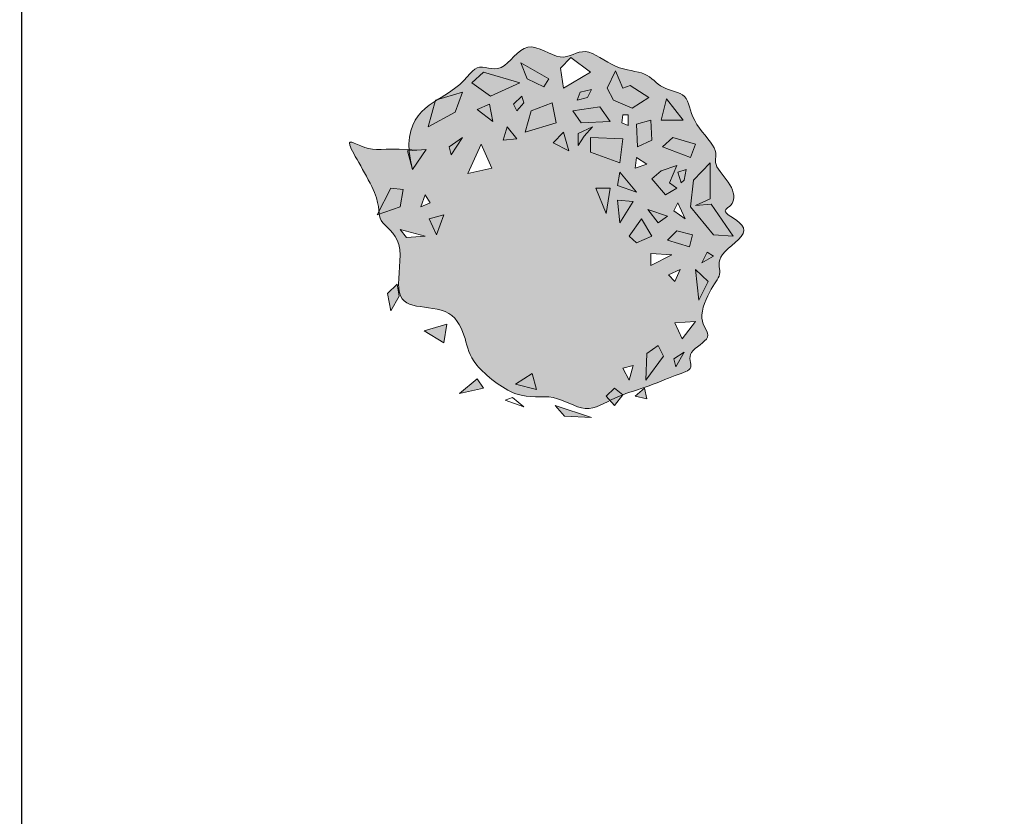
# Model space of a CAD drawing. Units: metres. Extents: x 4298.5 to 4325.2, y 2075 to 2095.8.
# Tile 29 of 35: x 4320.314 to 4321.936, y 2082.247 to 2083.561. Entities that reach past the tile are written whole.
import ezdxf

# ---------------------------------------------------------------- set-up
doc = ezdxf.new("R2010")
doc.units = ezdxf.units.M
doc.layers.add('A-ANNO-DIMS', color=2, linetype='Continuous', lineweight=18)
doc.layers.add('L-PLNT', color=94, linetype='Continuous', lineweight=13)
doc.layers.add('L-PLNT-PATT', color=116, linetype='Continuous', lineweight=13, true_color=0x13823e)
doc.styles.get("Standard").update_dxf_attribs({"font": 'arial.ttf'})
doc.dimstyles.get("Standard").update_dxf_attribs({"dimtxt": 0.18, "dimasz": 0.18, "dimexe": 0.18, "dimexo": 0.0625, "dimgap": 0.09, "dimtad": 0, "dimtih": 1, "dimtoh": 1, "dimdec": 4, "dimzin": 0, "dimdsep": 46, "dimtxsty": 'Standard', "dimcen": 0.09, "dimadec": 0, "dimazin": 0, "dimtfac": 1, "dimtdec": 4, "dimtofl": 0, "dimtmove": 0, "dimatfit": 3, "dimfxl": 1, "dimtolj": 1, "dimtzin": 0, "dimarcsym": 0})

# ---------------------------------------------------------------- blocks, each defined once
blk = doc.blocks.new('*U9')
for points in [[(-2.003, 11.656), (-1.598, 10.618), (-0.518, 10.099), (-0.181, 10.618), (-0.788, 10.964)], [(1.237, 12.003), (0.562, 11.31), (0.764, 10.013), (2.519, 11.051)], [(-4.432, 11.051), (-5.175, 10.359), (-3.96, 9.493), (-2.07, 10.359)], [(4.139, 11.137), (3.599, 10.013), (4.004, 9.234), (5.218, 8.715), (6.298, 9.407), (5.083, 10.186), (4.611, 10.013)], [(-5.782, 9.753), (-7.537, 9.234), (-8.009, 7.504), (-6.255, 8.455)], [(2.586, 9.926), (1.844, 9.753), (1.642, 9.234), (2.316, 9.407)], [(-4.837, 8.628), (-3.825, 7.85), (-4.027, 8.974)], [(-1.935, 9.493), (-2.475, 8.974), (-2.273, 8.542), (-1.8, 9.061)], [(0.022, 9.061), (-1.328, 8.542), (-1.733, 7.157), (0.292, 7.763)], [(7.446, 9.32), (7.108, 7.936), (8.525, 7.936)], [(1.372, 8.542), (3.126, 8.801), (3.801, 7.85), (1.912, 7.763)], [(4.611, 8.282), (4.544, 7.763), (4.949, 7.59), (4.949, 8.282)], [(6.433, 7.936), (5.488, 7.676), (5.556, 6.206), (6.501, 6.638)], [(-2.88, 7.504), (-3.15, 6.638), (-2.273, 6.725)], [(0.764, 7.157), (0.089, 6.465), (1.102, 5.946)], [(1.709, 6.292), (1.709, 7.071), (2.654, 7.504), (2.114, 6.898)], [(-5.782, 6.811), (-6.659, 6.206), (-6.524, 5.687)], [(2.519, 6.811), (2.519, 5.86), (4.409, 5.167), (4.611, 6.725)], [(7.851, 6.811), (7.176, 6.206), (8.998, 5.514), (9.335, 6.379)], [(-8.144, 6.033), (-9.359, 5.946), (-9.022, 4.735)], [(-4.567, 6.379), (-5.445, 4.475), (-3.892, 4.821)], [(5.488, 5.514), (5.421, 4.821), (6.163, 5.081)], [(10.28, 5.167), (9.2, 4.043), (8.998, 2.312), (10.482, 0.495), (11.765, 0.409), (10.348, 2.485), (9.335, 2.399), (10.28, 2.831)], [(4.409, 4.562), (4.274, 3.697), (5.488, 3.264)], [(8.12, 4.994), (7.108, 4.648), (6.501, 4.129), (7.378, 3.091), (8.12, 3.524), (7.648, 3.87)], [(8.728, 4.735), (8.188, 4.562), (8.39, 3.87), (8.593, 4.043)], [(-11.316, 1.793), (-9.831, 2.312), (-9.629, 3.437), (-10.439, 3.524)], [(3.531, 1.88), (2.856, 3.524), (3.801, 3.524)], [(-8.212, 3.091), (-8.482, 2.312), (-7.874, 2.572)], [(4.274, 2.745), (5.286, 2.658), (4.409, 1.274)], [(8.188, 2.572), (7.918, 2.053), (8.66, 1.534)], [(7.513, 1.707), (6.906, 1.274), (6.231, 2.139)], [(-6.997, 1.793), (-7.942, 1.534), (-7.469, 0.495)], [(5.826, 1.534), (5.016, 0.409), (5.488, -0.024), (6.501, 0.409)], [(-8.212, 0.409), (-9.426, 0.322), (-9.831, 0.841)], [(8.12, 0.755), (7.513, 0.149), (8.93, -0.283), (9.133, 0.495)], [(10.078, -0.629), (9.74, -1.322), (10.482, -0.889)], [(7.783, -0.803), (6.433, -1.495), (6.433, -0.716)], [(8.323, -1.754), (7.985, -2.533), (7.581, -2.1)], [(9.335, -1.754), (9.538, -3.744), (10.145, -2.533)], [(-10.034, -2.706), (-10.641, -3.312), (-10.439, -4.436), (-9.899, -3.485)], [(-8.279, -5.734), (-6.794, -5.302), (-6.997, -6.513)], [(9.335, -5.129), (8.458, -6.253), (7.985, -5.215)], [(6.096, -8.935), (6.163, -7.205), (6.906, -6.686), (7.243, -7.378)], [(8.053, -8.07), (8.593, -7.118), (7.918, -7.551)], [(5.286, -7.984), (4.611, -8.157), (5.016, -8.935)], [(-4.837, -8.849), (-4.432, -9.454), (-5.985, -9.801)], [(-2.34, -9.195), (-1.26, -8.503), (-0.99, -9.541)], [(4.071, -9.454), (3.531, -9.974), (4.071, -10.579), (4.611, -9.887)], [(6.028, -9.454), (5.421, -9.974), (6.163, -10.147)], [(-2.543, -10.06), (-3.015, -10.233), (-1.8, -10.666)], [(0.224, -10.579), (0.832, -11.272), (2.586, -11.358)]]:
    blk.add_lwpolyline(points, close=True)
blk = doc.blocks.new('*D47')
at = {"layer": 'A-ANNO-DIMS', "color": 0, "lineweight": -2, "transparency": 16777216}
for p, q in [((4300.4306, 2084.4956), (4300.4306, 2074.9896)), ((4322.8106, 2084.4956), (4322.8106, 2074.9896)), ((4300.6106, 2075.1696), (4311.2252, 2075.1696)), ((4322.6306, 2075.1696), (4312.016, 2075.1696))]:
    blk.add_line(p, q, dxfattribs=at)
at = {"layer": 'A-ANNO-DIMS', "color": 0, "transparency": 16777216}
for points in [[(4300.6106, 2075.1996), (4300.6106, 2075.1396), (4300.4306, 2075.1696)], [(4322.6306, 2075.1996), (4322.6306, 2075.1396), (4322.8106, 2075.1696)]]:
    blk.add_solid(points, dxfattribs=at)
at = {"layer": 'Defpoints', "color": 0, "transparency": 16777216}
for p in [(4300.4306, 2084.5581), (4322.8106, 2084.5581), (4322.8106, 2075.1696)]:
    blk.add_point(p, dxfattribs=at)
at = {"layer": 'A-ANNO-DIMS', "color": 0, "transparency": 16777216, "insert": (4311.6206, 2075.1696), "char_height": 0.18, "attachment_point": 5}
blk.add_mtext('\\A1;22.38', dxfattribs=at)
blk = doc.blocks.new('*D48')
at = {"layer": 'A-ANNO-DIMS', "color": 0, "lineweight": -2, "transparency": 16777216}
for p, q in [((4310.1831, 2094.4781), (4324.7671, 2094.4781)), ((4324.5871, 2094.2981), (4324.5871, 2085.585)), ((4324.5871, 2076.5081), (4324.5871, 2085.2212)), ((4316.8731, 2076.3281), (4324.7671, 2076.3281))]:
    blk.add_line(p, q, dxfattribs=at)
at = {"layer": 'A-ANNO-DIMS', "color": 0, "transparency": 16777216}
for points in [[(4324.5571, 2094.2981), (4324.6171, 2094.2981), (4324.5871, 2094.4781)], [(4324.5571, 2076.5081), (4324.6171, 2076.5081), (4324.5871, 2076.3281)]]:
    blk.add_solid(points, dxfattribs=at)
at = {"layer": 'Defpoints', "color": 0, "transparency": 16777216}
for p in [(4310.1206, 2094.4781), (4316.8106, 2076.3281), (4324.5871, 2076.3281)]:
    blk.add_point(p, dxfattribs=at)
at = {"layer": 'A-ANNO-DIMS', "color": 0, "transparency": 16777216, "insert": (4324.5871, 2085.4031), "char_height": 0.18, "attachment_point": 5}
blk.add_mtext('\\A1;18.15', dxfattribs=at)
blk = doc.blocks.new('*D55')
at = {"layer": 'A-ANNO-DIMS', "color": 0, "lineweight": -2, "transparency": 16777216}
for p, q in [((4320.3167, 2084.4996), (4320.3167, 2074.9896)), ((4322.8106, 2084.4956), (4322.8106, 2074.9896)), ((4320.4967, 2075.1696), (4321.1688, 2075.1696)), ((4322.6306, 2075.1696), (4321.9585, 2075.1696))]:
    blk.add_line(p, q, dxfattribs=at)
at = {"layer": 'A-ANNO-DIMS', "color": 0, "transparency": 16777216}
for points in [[(4320.4967, 2075.1996), (4320.4967, 2075.1396), (4320.3167, 2075.1696)], [(4322.6306, 2075.1996), (4322.6306, 2075.1396), (4322.8106, 2075.1696)]]:
    blk.add_solid(points, dxfattribs=at)
at = {"layer": 'Defpoints', "color": 0, "transparency": 16777216}
for p in [(4320.3167, 2084.5621), (4322.8106, 2084.5581), (4322.8106, 2075.1696)]:
    blk.add_point(p, dxfattribs=at)
at = {"layer": 'A-ANNO-DIMS', "color": 0, "transparency": 16777216, "insert": (4321.5636, 2075.1696), "char_height": 0.18, "attachment_point": 5}
blk.add_mtext('\\A1;2.494', dxfattribs=at)

msp = doc.modelspace()

# ---------------------------------------------------------------- hatches: boundary and pattern name
at = {"layer": 'L-PLNT-PATT'}
h = msp.add_hatch(color=256, dxfattribs=at)
h.dxf.hatch_style = 1
edge = h.paths.add_edge_path()
edge.add_spline(control_points=[(4321.2862, 2082.9328), (4321.2888, 2082.9341), (4321.3075, 2082.9435), (4321.3433, 2082.9532), (4321.3978, 2082.9765), (4321.4271, 2082.9841), (4321.4084, 2083.0126), (4321.461, 2083.0368), (4321.4273, 2083.0631), (4321.4543, 2083.1228), (4321.473, 2083.1423), (4321.4564, 2083.1708), (4321.5306, 2083.2156), (4321.4607, 2083.2452), (4321.4933, 2083.2529), (4321.4894, 2083.288), (4321.4513, 2083.3246), (4321.4698, 2083.3439), (4321.4168, 2083.3949), (4321.4168, 2083.441), (4321.3689, 2083.4443), (4321.3485, 2083.4762), (4321.2953, 2083.4762), (4321.2429, 2083.5216), (4321.2082, 2083.4845), (4321.1475, 2083.5353), (4321.1076, 2083.4653), (4321.063, 2083.4952), (4321.0487, 2083.4559), (4321.0084, 2083.4328), (4321.002, 2083.4289)], knot_values=[0.818571, 0.818571, 0.818571, 0.818571, 0.97924, 1.97924, 2.97924, 3.97924, 4.97924, 5.97924, 6.97924, 7.97924, 8.97924, 9.97924, 10.97924, 11.97924, 12.97924, 13.97924, 14.97924, 15.97924, 16.97924, 17.97924, 18.97924, 19.97924, 20.97924, 21.97924, 22.97924, 23.97924, 24.97924, 25.97924, 26.97924, 27.16067, 27.16067, 27.16067, 27.16067], degree=3, periodic=0)
edge.add_line((4321.002, 2083.4289), (4321.0433, 2083.4411))
edge.add_line((4321.0433, 2083.4411), (4321.0313, 2083.4081))
edge.add_line((4321.0313, 2083.4081), (4320.9867, 2083.384))
edge.add_line((4320.9867, 2083.384), (4320.9983, 2083.4265))
edge.add_spline(control_points=[(4320.9983, 2083.4265), (4320.9757, 2083.4119), (4320.9524, 2083.3909), (4320.9551, 2083.3465)], knot_values=[0.141368, 0.141368, 0.141368, 0.141368, 0.783694, 0.783694, 0.783694, 0.783694], degree=3, periodic=0)
edge.add_spline(control_points=[(4320.9551, 2083.3465), (4320.9591, 2083.3463), (4320.9633, 2083.3459), (4320.9679, 2083.3455)], knot_values=[40.901028, 40.901028, 40.901028, 40.901028, 41, 41, 41, 41], degree=3, periodic=0)
edge.add_line((4320.9679, 2083.3455), (4320.9833, 2083.3466))
edge.add_line((4320.9833, 2083.3466), (4320.961, 2083.3136))
edge.add_line((4320.961, 2083.3136), (4320.9524, 2083.3444))
edge.add_line((4320.9524, 2083.3444), (4320.9552, 2083.3446))
edge.add_spline(control_points=[(4320.9553, 2083.3446), (4320.9552, 2083.3452), (4320.9552, 2083.3459), (4320.9551, 2083.3465)], knot_values=[0.13204, 0.13204, 0.13204, 0.13204, 0.141368, 0.141368, 0.141368, 0.141368], degree=3, periodic=0)
edge.add_spline(control_points=[(4320.9551, 2083.3465), (4320.9189, 2083.3489), (4320.8873, 2083.339), (4320.8353, 2083.381), (4320.9023, 2083.2785), (4320.9047, 2083.2516), (4320.9054, 2083.2441)], knot_values=[37.439141, 37.439141, 37.439141, 37.439141, 38.340169, 39.340169, 40.340169, 40.901028, 40.901028, 40.901028, 40.901028], degree=3, periodic=0)
edge.add_line((4320.9054, 2083.2441), (4320.925, 2083.2829))
edge.add_line((4320.925, 2083.2829), (4320.9456, 2083.2807))
edge.add_line((4320.9456, 2083.2807), (4320.9404, 2083.2521))
edge.add_line((4320.9404, 2083.2521), (4320.9058, 2083.24))
edge.add_spline(control_points=[(4320.9058, 2083.24), (4320.9063, 2083.236), (4320.9094, 2083.2225), (4320.9507, 2083.2015), (4320.9293, 2083.1043), (4320.9615, 2083.0854), (4321.0277, 2083.0854), (4321.0505, 2083.0317), (4321.054, 2082.9962), (4321.135, 2082.9301), (4321.1933, 2082.9469), (4321.2437, 2082.91), (4321.2728, 2082.926), (4321.2862, 2082.9328)], knot_values=[27.16067, 27.16067, 27.16067, 27.16067, 27.490087, 28.490087, 29.490087, 30.490087, 31.490087, 32.490087, 33.490087, 34.490087, 35.490087, 36.490087, 37.329418, 37.329418, 37.329418, 37.329418], degree=3, periodic=0)
edge.add_line((4321.2862, 2082.9328), (4321.2798, 2082.94))
edge.add_line((4321.2798, 2082.94), (4321.2935, 2082.9532))
edge.add_line((4321.2935, 2082.9532), (4321.3073, 2082.9422))
h.paths.add_polyline_path([(4321.2627, 2083.2829), (4321.2867, 2083.2829), (4321.2798, 2083.2411)], flags=16)
h.paths.add_polyline_path([(4321.2987, 2083.2631), (4321.3244, 2083.2609), (4321.3021, 2083.2257)], flags=16)
h.paths.add_polyline_path([(4321.0913, 2083.3158), (4321.0518, 2083.307), (4321.0741, 2083.3554)], flags=16)
h.paths.add_polyline_path([(4321.2181, 2083.3444), (4321.1924, 2083.3576), (4321.2095, 2083.3751)], flags=16)
h.paths.add_polyline_path([(4321.2987, 2083.2873), (4321.3021, 2083.3092), (4321.3295, 2083.2763)], flags=16)
h.paths.add_polyline_path([(4321.3175, 2083.2037), (4321.3381, 2083.2323), (4321.3553, 2083.2037), (4321.3295, 2083.1927)], flags=16)
h.paths.add_polyline_path([(4321.2541, 2083.3422), (4321.2541, 2083.3664), (4321.3073, 2083.3642), (4321.3021, 2083.3246)], flags=16)
h.paths.add_polyline_path([(4321.2335, 2083.3532), (4321.2335, 2083.373), (4321.2576, 2083.384), (4321.2438, 2083.3686)], flags=16)
h.paths.add_polyline_path([(4321.1324, 2083.3642), (4321.1101, 2083.362), (4321.117, 2083.384)], flags=16)
h.paths.add_polyline_path([(4321.1461, 2083.3751), (4321.1564, 2083.4103), (4321.1907, 2083.4235), (4321.1976, 2083.3905)], flags=16)
h.paths.add_polyline_path([(4321.0124, 2083.2389), (4321.0004, 2083.2059), (4320.9884, 2083.2323)], flags=16)
h.paths.add_polyline_path([(4321.3484, 2083.2477), (4321.381, 2083.2367), (4321.3656, 2083.2257)], flags=16)
h.paths.add_polyline_path([(4321.3278, 2083.3158), (4321.3295, 2083.3334), (4321.3467, 2083.3224)], flags=16)
h.paths.add_polyline_path([(4321.2387, 2083.3905), (4321.225, 2083.4103), (4321.2695, 2083.4169), (4321.2867, 2083.3927)], flags=16)
h.paths.add_polyline_path([(4321.3535, 2083.1752), (4321.3878, 2083.173), (4321.3535, 2083.1554)], flags=16)
h.paths.add_polyline_path([(4320.9901, 2083.2587), (4320.9747, 2083.2521), (4320.9816, 2083.2719)], flags=16)
h.paths.add_polyline_path([(4321.093, 2083.3927), (4321.0673, 2083.4125), (4321.0879, 2083.4213)], flags=16)
h.paths.add_polyline_path([(4321.0244, 2083.3378), (4321.021, 2083.351), (4321.0433, 2083.3664)], flags=16)
h.paths.add_polyline_path([(4321.1324, 2083.4103), (4321.1273, 2083.4213), (4321.141, 2083.4345), (4321.1444, 2083.4235)], flags=16)
h.paths.add_polyline_path([(4321.3553, 2083.2982), (4321.3707, 2083.3114), (4321.3964, 2083.3202), (4321.3844, 2083.2917), (4321.3964, 2083.2829), (4321.3775, 2083.2719)], flags=16)
h.paths.add_polyline_path([(4320.9816, 2083.2037), (4320.9507, 2083.2015), (4320.9404, 2083.2147)], flags=16)
h.paths.add_polyline_path([(4321.3313, 2083.351), (4321.3295, 2083.3883), (4321.3535, 2083.3949), (4321.3553, 2083.362)], flags=16)
h.paths.add_polyline_path([(4321.381, 2083.1971), (4321.3964, 2083.2125), (4321.4221, 2083.2059), (4321.417, 2083.1862)], flags=16)
h.paths.add_polyline_path([(4321.3056, 2083.3905), (4321.3073, 2083.4037), (4321.3158, 2083.4037), (4321.3158, 2083.3861)], flags=16)
h.paths.add_polyline_path([(4321.2318, 2083.4279), (4321.237, 2083.4411), (4321.2558, 2083.4455), (4321.249, 2083.4323)], flags=16)
h.paths.add_polyline_path([(4321.3913, 2083.2455), (4321.3981, 2083.2587), (4321.4101, 2083.2323)], flags=16)
h.paths.add_polyline_path([(4321.3827, 2083.14), (4321.4015, 2083.1488), (4321.393, 2083.129)], flags=16)
h.paths.add_polyline_path([(4321.177, 2083.4499), (4321.1496, 2083.4631), (4321.1393, 2083.4894), (4321.1701, 2083.4718), (4321.1855, 2083.4631)], flags=16)
h.paths.add_polyline_path([(4321.2095, 2083.4477), (4321.2044, 2083.4806), (4321.2216, 2083.4982), (4321.2541, 2083.4741)], flags=16)
h.paths.add_polyline_path([(4321.0896, 2083.4345), (4321.0587, 2083.4565), (4321.0776, 2083.4741), (4321.1376, 2083.4565)], flags=16)
h.paths.add_polyline_path([(4321.3724, 2083.351), (4321.3896, 2083.3664), (4321.4273, 2083.3554), (4321.4187, 2083.3334)], flags=16)
h.paths.add_polyline_path([(4321.2918, 2083.4279), (4321.2816, 2083.4477), (4321.2953, 2083.4762), (4321.3073, 2083.4477), (4321.3192, 2083.4521), (4321.3501, 2083.4323), (4321.3227, 2083.4147)], flags=16)
h.paths.add_polyline_path([(4321.4032, 2083.2917), (4321.3981, 2083.3092), (4321.4118, 2083.3136), (4321.4084, 2083.2961)], flags=16)
h.paths.add_polyline_path([(4321.4187, 2083.2521), (4321.4238, 2083.2961), (4321.4513, 2083.3246), (4321.4513, 2083.2653), (4321.4273, 2083.2543), (4321.453, 2083.2565), (4321.489, 2083.2037), (4321.4564, 2083.2059)], flags=16)
h.paths.add_polyline_path([(4321.1581, 2082.9774), (4321.165, 2082.951), (4321.1307, 2082.9598)], flags=16)
h.paths.add_polyline_path([(4321.3707, 2083.3949), (4321.3793, 2083.4301), (4321.4067, 2083.3949)], flags=16)
h.paths.add_polyline_path([(4321.4273, 2083.1488), (4321.4478, 2083.129), (4321.4324, 2083.0983)], flags=16)
h.paths.add_polyline_path([(4321.4375, 2083.1598), (4321.4461, 2083.1774), (4321.4564, 2083.1708)], flags=16)
h.paths.add_polyline_path([(4321.3073, 2082.9862), (4321.3244, 2082.9906), (4321.3175, 2082.9664)], flags=16)
h.paths.add_polyline_path([(4321.393, 2083.0609), (4321.4273, 2083.0631), (4321.405, 2083.0345)], flags=16)
h.paths.add_polyline_path([(4321.3467, 2083.0104), (4321.3656, 2083.0235), (4321.3741, 2083.006), (4321.345, 2082.9664)], flags=16)
h.paths.add_polyline_path([(4321.3913, 2083.0016), (4321.4084, 2083.0126), (4321.3947, 2082.9884)], flags=16)
h = msp.add_hatch(color=256, dxfattribs=at)
h.dxf.hatch_style = 1
h.paths.add_polyline_path([(4321.3021, 2083.3246), (4321.3073, 2083.3642), (4321.2541, 2083.3664), (4321.2541, 2083.3422)])
h.paths.add_polyline_path([(4321.3484, 2083.2477), (4321.3656, 2083.2257), (4321.381, 2083.2367)])
h.paths.add_polyline_path([(4321.3295, 2083.3883), (4321.3313, 2083.351), (4321.3553, 2083.362), (4321.3535, 2083.3949)])
h.paths.add_polyline_path([(4321.3501, 2083.4323), (4321.3192, 2083.4521), (4321.3073, 2083.4477), (4321.2953, 2083.4762), (4321.2816, 2083.4477), (4321.2918, 2083.4279), (4321.3227, 2083.4147)])
h.paths.add_polyline_path([(4321.1958, 2082.9247), (4321.2113, 2082.907), (4321.2558, 2082.9049)])
h.paths.add_polyline_path([(4321.177, 2083.4499), (4321.1855, 2083.4631), (4321.1701, 2083.4718), (4321.1393, 2083.4894), (4321.1496, 2083.4631)])
h.paths.add_polyline_path([(4321.0776, 2083.4741), (4321.0587, 2083.4565), (4321.0896, 2083.4345), (4321.1376, 2083.4565)])
h.paths.add_polyline_path([(4321.1564, 2083.4103), (4321.1461, 2083.3751), (4321.1976, 2083.3905), (4321.1907, 2083.4235)])
h.paths.add_polyline_path([(4321.1444, 2083.4235), (4321.141, 2083.4345), (4321.1273, 2083.4213), (4321.1324, 2083.4103)])
h.paths.add_polyline_path([(4321.117, 2083.384), (4321.1101, 2083.362), (4321.1324, 2083.3642)])
h.paths.add_polyline_path([(4321.093, 2083.3927), (4321.0879, 2083.4213), (4321.0673, 2083.4125)])
h.paths.add_polyline_path([(4320.9987, 2083.4279), (4320.9867, 2083.384), (4321.0313, 2083.4081), (4321.0433, 2083.4411)])
h.paths.add_polyline_path([(4321.0433, 2083.3664), (4321.021, 2083.351), (4321.0244, 2083.3378)])
h.paths.add_polyline_path([(4320.9524, 2083.3444), (4320.961, 2083.3136), (4320.9833, 2083.3466)])
h.paths.add_polyline_path([(4320.9027, 2083.2389), (4320.9404, 2083.2521), (4320.9456, 2083.2807), (4320.925, 2083.2829)])
h.paths.add_polyline_path([(4321.0124, 2083.2389), (4320.9884, 2083.2323), (4321.0004, 2083.2059)])
h.paths.add_polyline_path([(4320.9387, 2083.1048), (4320.9353, 2083.1246), (4320.9199, 2083.1092), (4320.925, 2083.0807)])
h.paths.add_polyline_path([(4321.0176, 2083.0587), (4320.9799, 2083.0477), (4321.0124, 2083.0279)])
h.paths.add_polyline_path([(4321.0381, 2082.9444), (4321.0776, 2082.9532), (4321.0673, 2082.9686)])
h.paths.add_polyline_path([(4321.1581, 2082.9774), (4321.1307, 2082.9598), (4321.165, 2082.951)])
h.paths.add_polyline_path([(4321.2935, 2082.9532), (4321.2798, 2082.94), (4321.2935, 2082.9247), (4321.3073, 2082.9422)])
h.paths.add_polyline_path([(4321.3741, 2083.006), (4321.3656, 2083.0235), (4321.3467, 2083.0104), (4321.345, 2082.9664)])
h.paths.add_polyline_path([(4321.3433, 2082.9532), (4321.3278, 2082.94), (4321.3467, 2082.9356)])
h.paths.add_polyline_path([(4321.3913, 2083.0016), (4321.3947, 2082.9884), (4321.4084, 2083.0126)])
h.paths.add_polyline_path([(4321.4324, 2083.0983), (4321.4478, 2083.129), (4321.4273, 2083.1488)])
h.paths.add_polyline_path([(4321.3175, 2083.2037), (4321.3295, 2083.1927), (4321.3553, 2083.2037), (4321.3381, 2083.2323)])
h.paths.add_polyline_path([(4321.4564, 2083.2059), (4321.489, 2083.2037), (4321.453, 2083.2565), (4321.4273, 2083.2543), (4321.4513, 2083.2653), (4321.4513, 2083.3246), (4321.4238, 2083.2961), (4321.4187, 2083.2521)])
h.paths.add_polyline_path([(4321.3964, 2083.2125), (4321.381, 2083.1971), (4321.417, 2083.1862), (4321.4221, 2083.2059)])
h.paths.add_polyline_path([(4321.4564, 2083.1708), (4321.4461, 2083.1774), (4321.4375, 2083.1598)])
h.paths.add_polyline_path([(4321.3964, 2083.3202), (4321.3707, 2083.3114), (4321.3553, 2083.2982), (4321.3775, 2083.2719), (4321.3964, 2083.2829), (4321.3844, 2083.2917)])
h.paths.add_polyline_path([(4321.3981, 2083.3092), (4321.4032, 2083.2917), (4321.4084, 2083.2961), (4321.4118, 2083.3136)])
h.paths.add_polyline_path([(4321.4187, 2083.3334), (4321.4273, 2083.3554), (4321.3896, 2083.3664), (4321.3724, 2083.351)])
h.paths.add_polyline_path([(4321.3295, 2083.2763), (4321.3021, 2083.3092), (4321.2987, 2083.2873)])
h.paths.add_polyline_path([(4321.2867, 2083.2829), (4321.2627, 2083.2829), (4321.2798, 2083.2411)])
h.paths.add_polyline_path([(4321.3244, 2083.2609), (4321.2987, 2083.2631), (4321.3021, 2083.2257)])
h.paths.add_polyline_path([(4321.2867, 2083.3927), (4321.2695, 2083.4169), (4321.225, 2083.4103), (4321.2387, 2083.3905)])
h.paths.add_polyline_path([(4321.2438, 2083.3686), (4321.2576, 2083.384), (4321.2335, 2083.373), (4321.2335, 2083.3532)])
h.paths.add_polyline_path([(4321.2095, 2083.3751), (4321.1924, 2083.3576), (4321.2181, 2083.3444)])
h.paths.add_polyline_path([(4321.249, 2083.4323), (4321.2558, 2083.4455), (4321.237, 2083.4411), (4321.2318, 2083.4279)])
h.paths.add_polyline_path([(4321.3793, 2083.4301), (4321.3707, 2083.3949), (4321.4067, 2083.3949)])

# ---------------------------------------------------------------- linework, layer by layer
at = {"layer": 'L-PLNT'}
msp.add_open_spline([(4320.961, 2083.3136), (4320.9369, 2083.4001), (4321.0433, 2083.4411), (4321.063, 2083.4952), (4321.1076, 2083.4653), (4321.1475, 2083.5353), (4321.2082, 2083.4845), (4321.2429, 2083.5216), (4321.2953, 2083.4762), (4321.3485, 2083.4762), (4321.3689, 2083.4443), (4321.4168, 2083.441), (4321.4168, 2083.3949), (4321.4698, 2083.3439), (4321.4513, 2083.3246), (4321.4894, 2083.288), (4321.4933, 2083.2529), (4321.4607, 2083.2452), (4321.5306, 2083.2156), (4321.4564, 2083.1708), (4321.473, 2083.1423), (4321.4543, 2083.1228), (4321.4273, 2083.0631), (4321.461, 2083.0368), (4321.4084, 2083.0126), (4321.4271, 2082.9841), (4321.3978, 2082.9765), (4321.3433, 2082.9532), (4321.2935, 2082.9397), (4321.2465, 2082.9079), (4321.1933, 2082.9469), (4321.135, 2082.9301), (4321.054, 2082.9962), (4321.0505, 2083.0317), (4321.0277, 2083.0854), (4320.9615, 2083.0854), (4320.9293, 2083.1043), (4320.9507, 2083.2015), (4320.8975, 2083.2285), (4320.9139, 2083.2609), (4320.8353, 2083.381), (4320.8891, 2083.3376), (4320.9222, 2083.35), (4320.9679, 2083.3455)], degree=3, dxfattribs=at)

# ---------------------------------------------------------------- block references
at = {"layer": 'L-PLNT', "xscale": 0.0254, "yscale": 0.0254, "zscale": 0.0254}
msp.add_blockref('*U9', (4321.1901, 2083.1934), dxfattribs=at)

# ---------------------------------------------------------------- dimensions: what is measured, and where the dimension line sits
at = {"layer": 'A-ANNO-DIMS'}
dim = msp.add_linear_dim(base=(4324.5871, 2076.3281), p1=(4310.1206, 2094.4781), p2=(4316.8106, 2076.3281), angle=90, dimstyle='Standard', override={"dimdec": 2, "dimlfac": 1, "dimrnd": 0, "dimzin": 0, "dimdsep": 46, "dimlunit": 2}, dxfattribs=at)
dim.commit()
dim.dimension.update_dxf_attribs({"geometry": '*D48', "text_midpoint": (4324.5871, 2085.4031)})
for p1, override, picture, middle in [((4300.4306, 2084.5581), {"dimdec": 2, "dimlfac": 1, "dimrnd": 0, "dimzin": 0, "dimdsep": 46, "dimlunit": 2}, '*D47', (4311.6206, 2075.1696)), ((4320.3167, 2084.5621), {"dimdec": 3, "dimlfac": 1, "dimrnd": 0, "dimzin": 0, "dimdsep": 46, "dimlunit": 2}, '*D55', (4321.5636, 2075.1696))]:
    dim = msp.add_linear_dim(base=(4322.8106, 2075.1696), p1=p1, p2=(4322.8106, 2084.5581), dimstyle='Standard', override=override, dxfattribs=at)
    dim.commit()
    dim.dimension.update_dxf_attribs({"geometry": picture, "text_midpoint": middle})

doc.saveas('drawing.dxf')
